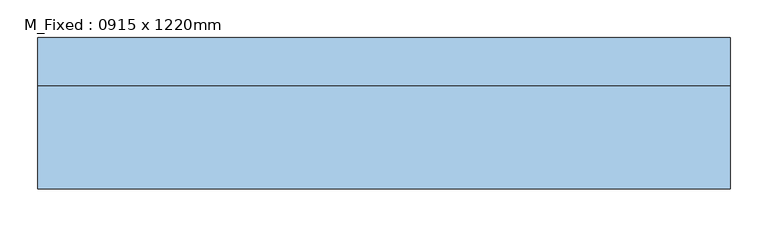
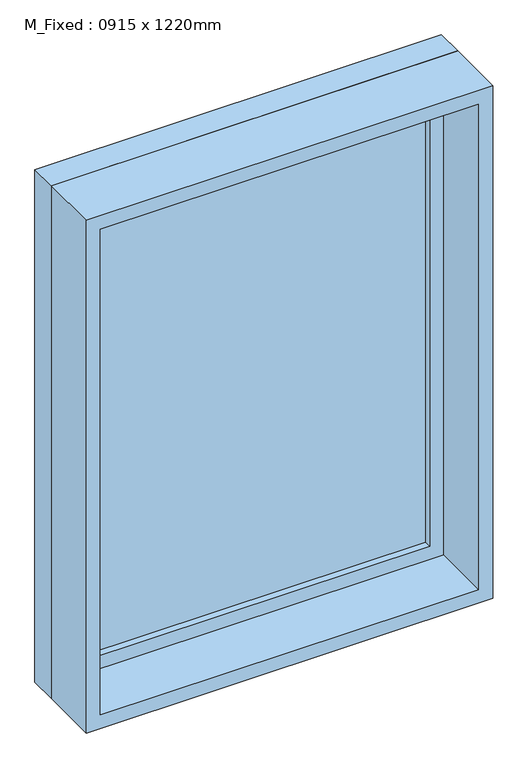
"""IFC4 building model written with IfcOpenShell, lengths in millimetres: window geometry, M_Fixed : 0915 x 1220mm."""

from ifc_helpers import new_model, si_unit, frame, origin, place, context, project, spatial, polyline, outline, extrude, source, transform, mapped, element, save


def m_fixed_0915_x_1220mm_488fb2fb(model_context):
    return source(origin(), model_context, "Body", "SweptSolid", [
        extrude(outline(polyline([(-394.5, 78.0), (394.5, 78.0), (394.5, 66.0), (-394.5, 66.0), (-394.5, 78.0)])), frame((0.0, 0.0, 978.0), z_axis=(0.0, 0.0, 1.0), x_axis=(1.0, 0.0, 0.0)), (0.0, 0.0, 1.0), 1094.0),
        extrude(outline(polyline([(2116.0, -438.5), (934.0, -438.5), (934.0, 438.5), (2116.0, 438.5), (2116.0, -438.5)]), holes=[polyline([(2072.0, -394.5), (2072.0, 394.5), (978.0, 394.5), (978.0, -394.5), (2072.0, -394.5)])]), frame((0.0, 50.0, 0.0), z_axis=(0.0, 1.0, 0.0), x_axis=(0.0, 0.0, 1.0)), (0.0, 0.0, 1.0), 44.0),
        extrude(outline(polyline([(2135.0, -457.5), (915.0, -457.5), (915.0, 457.5), (2135.0, 457.5), (2135.0, -457.5)]), holes=[polyline([(2116.0, -438.5), (2116.0, 438.5), (934.0, 438.5), (934.0, -438.5), (2116.0, -438.5)])]), frame((0.0, 50.0, 0.0), z_axis=(0.0, 1.0, 0.0), x_axis=(0.0, 0.0, 1.0)), (0.0, 0.0, 1.0), 63.0),
        extrude(outline(polyline([(2135.0, -457.5), (915.0, -457.5), (915.0, 457.5), (2135.0, 457.5), (2135.0, -457.5)]), holes=[polyline([(2103.0, -425.5), (2103.0, 425.5), (947.0, 425.5), (947.0, -425.5), (2103.0, -425.5)])]), frame((0.0, -87.0, 0.0), z_axis=(0.0, 1.0, 0.0), x_axis=(0.0, 0.0, 1.0)), (0.0, 0.0, 1.0), 137.0),
    ])


if __name__ == "__main__":
    model = new_model("IFC4")
    model_context = context("Model", 3, world=origin())
    ifc_project = project(units=[si_unit("LENGTHUNIT", "METRE", prefix="MILLI")], contexts=[model_context])
    site = spatial("IfcSite", under=ifc_project)
    building = spatial("IfcBuilding", under=site)
    placement = place(None, origin())
    m_fixed_0915_x_1220mm_shape = m_fixed_0915_x_1220mm_488fb2fb(model_context)
    element("IfcWindow", 1, ObjectType="M_Fixed : 0915 x 1220mm", at=placement, inside=building, context=model_context, shape_type="MappedRepresentation", body=[
        mapped(m_fixed_0915_x_1220mm_shape, transform((0.0, 0.0, 0.0), x_axis=(1.0, 0.0, 0.0), y_axis=(0.0, 1.0, 0.0), z_axis=(0.0, 0.0, 1.0))),
    ])
    save(model, "model.ifc")

# Revit data of these elements
# Type "M_Fixed : 0915 x 1220mm"
#   Type Mark = "15"
#   Height = 4' - 0.0315"
#   Default Sill Height = 3' - 0.02362"
#   Width = 3' - 0.02362"
#   Window Inset = 0' - 0.74803"
#   Frame Exterior Material = Sash
#   Frame Interior Material = Sash
#   Glass Pane Material = Glass
#   Sash = Sash
#   Wall Closure = (empty or 0)
# Element 1 (IfcWindow, "M_Fixed : 0915 x 1220mm")
#   Materials on its faces: "Sash", "Glass"
# Materials
#   "Sash": class "Wood", colour RGB 136 99 55, transparency 0
#   "Glass": class "Glass", colour RGB 218 227 224, transparency 0.85, Description = "Soda Lime Glass", Cost = 0
